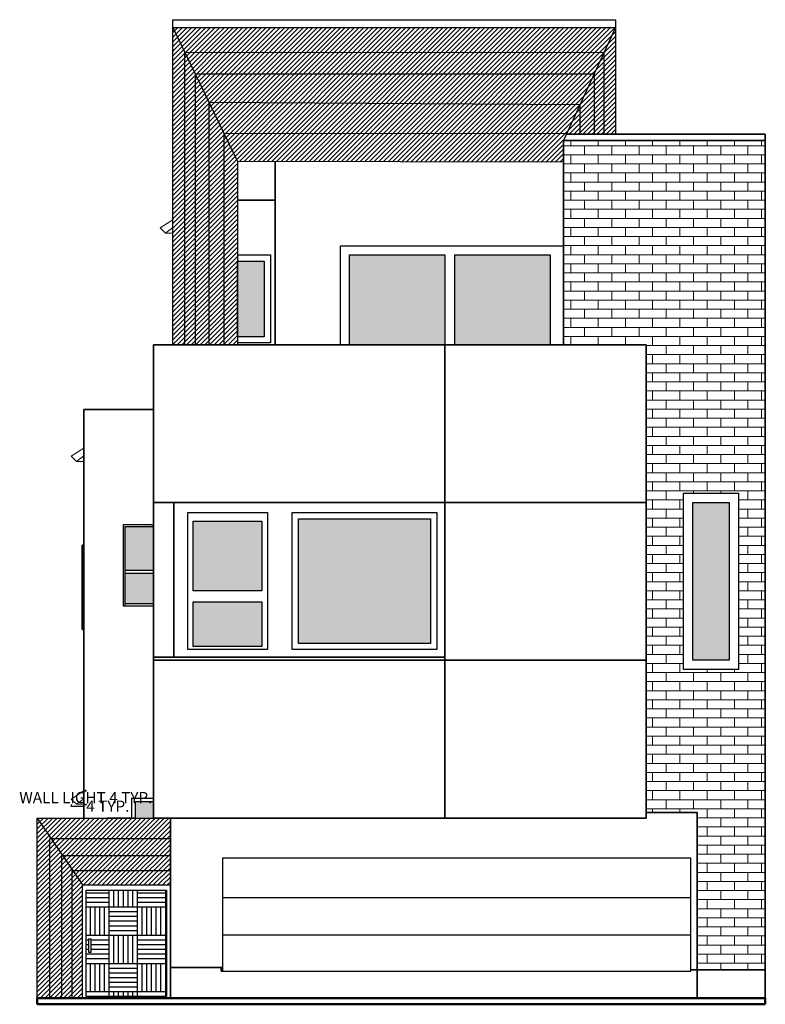
# Model space of a CAD drawing. Units: inches. Extents: x 236 to 476, y 69 to 387.
import ezdxf

# ---------------------------------------------------------------- set-up
doc = ezdxf.new("R2010")
doc.units = ezdxf.units.IN
doc.header["$MEASUREMENT"] = 0
for name, color, linetype, lineweight in [('A-ANNO-DIMS', 2, 'Continuous', 18), ('A-DOOR', 3, 'Continuous', 25), ('A-ELEV', 7, 'Continuous', 35), ('A-ELEV-FIXT', 9, 'Continuous', 18), ('A-ELEV-GRND', 7, 'Continuous', 50), ('A-GLAZ', 4, 'Continuous', 25), ('A-GLAZ-PATT', 251, 'Continuous', 13), ('A-ROOF', 1, 'Continuous', 25), ('A-ROOF-PATT', 8, 'Continuous', 13), ('A-WALL-PATT', 8, 'Continuous', 13)]:
    doc.layers.add(name, color=color, linetype=linetype, lineweight=lineweight)
doc.styles.get("Standard").update_dxf_attribs({"font": 'arial.ttf'})
doc.dimstyles.get("Standard").update_dxf_attribs({"dimtxt": 3.625, "dimasz": 0.18, "dimexe": 0.18, "dimexo": 0.0625, "dimgap": 0.09, "dimtad": 0, "dimtih": 1, "dimtoh": 1, "dimdec": 4, "dimzin": 0, "dimdsep": 46, "dimlunit": 4, "dimtxsty": 'Standard', "dimcen": 0.09, "dimadec": 0, "dimazin": 0, "dimtfac": 1, "dimtdec": 4, "dimtofl": 0, "dimtmove": 0, "dimatfit": 3, "dimfxl": 1, "dimtolj": 1, "dimtzin": 0, "dimarcsym": 0})

# ---------------------------------------------------------------- blocks, each defined once
blk = doc.blocks.new('WALL-LIGHT')
for p, q in [((0, 1.66), (4.13, 4.28)), ((1.8, 0), (0, 1.66)), ((4.13, 1.79), (1.8, 0)), ((1.8, 0), (4.13, 0))]:
    blk.add_line(p, q)
blk = doc.blocks.new('*D2')
at = {"layer": 'A-ANNO-DIMS', "color": 0, "lineweight": -2, "transparency": 16777216}
for p, q in [((256.36, 137.76), (257.12, 137.76)), ((256.94, 137.94), (256.94, 138.12)), ((256.36, 133.48), (257.12, 133.48)), ((256.94, 133.3), (256.94, 133.12))]:
    blk.add_line(p, q, dxfattribs=at)
at = {"layer": 'A-ANNO-DIMS', "color": 0, "transparency": 16777216}
for points in [[(256.91, 137.94), (256.97, 137.94), (256.94, 137.76)], [(256.91, 133.3), (256.97, 133.3), (256.94, 133.48)]]:
    blk.add_solid(points, dxfattribs=at)
at = {"layer": 'Defpoints', "color": 0, "transparency": 16777216}
for p in [(256.29, 137.76), (256.94, 137.76), (256.29, 133.48)]:
    blk.add_point(p, dxfattribs=at)
at = {"layer": 'A-ANNO-DIMS', "color": 0, "transparency": 16777216, "insert": (256.94, 135.62), "char_height": 3.625, "attachment_point": 5}
blk.add_mtext('\\A1;WALL LIGHT 4 TYP.', dxfattribs=at)
blk = doc.blocks.new('*D3')
at = {"layer": 'A-ANNO-DIMS', "color": 0, "lineweight": -2, "transparency": 16777216}
for p, q in [((252.16, 133.42), (252.16, 132.66)), ((252.34, 132.84), (256.11, 132.84)), ((256.29, 133.42), (256.29, 132.66)), ((256.29, 132.84), (256.47, 132.84))]:
    blk.add_line(p, q, dxfattribs=at)
at = {"layer": 'A-ANNO-DIMS', "color": 0, "transparency": 16777216}
for points in [[(252.34, 132.87), (252.34, 132.81), (252.16, 132.84)], [(256.11, 132.87), (256.11, 132.81), (256.29, 132.84)]]:
    blk.add_solid(points, dxfattribs=at)
at = {"layer": 'Defpoints', "color": 0, "transparency": 16777216}
for p in [(252.16, 133.48), (256.29, 133.48), (256.29, 132.84)]:
    blk.add_point(p, dxfattribs=at)
at = {"layer": 'A-ANNO-DIMS', "color": 0, "transparency": 16777216, "insert": (264.05, 132.84), "char_height": 3.625, "attachment_point": 5}
blk.add_mtext('\\A1;4 TYP.', dxfattribs=at)

msp = doc.modelspace()

# ---------------------------------------------------------------- hatches: boundary and pattern name
at = {"layer": 'A-DOOR'}
h = msp.add_hatch(dxfattribs=at)
h.set_pattern_fill('AR-PARQ1', color=256, scale=0.76)
h.paths.add_polyline_path([(283.03, 105.74), (257.04, 105.74), (257.04, 71.42), (283.03, 71.42)])
h.paths.add_polyline_path([(258.54, 89.96), (258.54, 85.61), (257.9, 85.61), (257.9, 89.96)], flags=16)
at = {"layer": 'A-GLAZ-PATT'}
h = msp.add_hatch(color=256, dxfattribs=at)
h.dxf.hatch_style = 1
h.paths.add_polyline_path([(372.93, 310.89), (342.13, 310.89), (342.13, 281.89), (372.93, 281.89)])
h.paths.add_polyline_path([(406.95, 310.89), (376.14, 310.89), (376.14, 281.89), (406.95, 281.89)])
h.paths.add_polyline_path([(368.29, 225.67), (325.59, 225.67), (325.59, 185.43), (368.29, 185.43)])
h.paths.add_polyline_path([(464.7, 230.94), (452.98, 230.94), (452.98, 179.98), (464.7, 179.98)])
h.paths.add_polyline_path([(314.54, 308.89), (305.89, 308.89), (305.89, 284.48), (314.54, 284.48)])
h.paths.add_polyline_path([(313.79, 224.94), (291.63, 224.94), (291.63, 202.39), (313.79, 202.39)])
h.paths.add_polyline_path([(313.79, 198.83), (291.63, 198.83), (291.63, 184.47), (313.79, 184.47)])
h.paths.add_polyline_path([(278.79, 223.2), (269.55, 223.2), (269.55, 209.06), (278.79, 209.06)])
h.paths.add_polyline_path([(278.79, 208.06), (269.55, 208.06), (269.55, 198.34), (278.79, 198.34)])
h.paths.add_polyline_path([(278.79, 134.31), (272.98, 134.31), (272.98, 129.02), (278.79, 129.02)])
at = {"layer": 'A-ROOF-PATT'}
h = msp.add_hatch(dxfattribs=at)
h.set_pattern_fill('ANSI31', color=256, scale=8.5)
h.paths.add_polyline_path([(245.32, 122.42), (245.67, 122.42), (241.2, 129.02), (241.2, 70.86), (245.32, 70.86)])
h.paths.add_polyline_path([(284.25, 129.02), (241.2, 129.02), (245.67, 122.42), (284.25, 122.42)])
h.paths.add_polyline_path([(284.25, 122.42), (245.67, 122.42), (249.39, 116.94), (284.25, 116.94)])
h.paths.add_polyline_path([(249.2, 116.94), (249.39, 116.94), (245.67, 122.42), (245.32, 122.42), (245.32, 70.86), (249.2, 70.86)])
h.paths.add_polyline_path([(252.56, 112.06), (252.71, 112.06), (249.39, 116.94), (249.2, 116.94), (249.2, 70.86), (252.56, 70.86)])
h.paths.add_polyline_path([(284.25, 116.94), (249.39, 116.94), (252.71, 112.06), (284.25, 112.06)])
h.paths.add_polyline_path([(284.25, 112.06), (252.71, 112.06), (255.87, 107.4), (284.25, 107.4)])
h.paths.add_polyline_path([(255.87, 107.4), (252.71, 112.06), (252.56, 112.06), (252.56, 70.86), (255.87, 70.86)])
h.paths.add_polyline_path([(411.16, 347.89), (412.27, 350.27), (301.56, 350.08), (305.89, 341.12), (411.16, 340.89)])
h.paths.add_polyline_path([(416.5, 359.44), (296.66, 360.24), (301.56, 350.08), (412.27, 350.27)])
h.paths.add_polyline_path([(421.09, 369.37), (292.24, 369.37), (296.66, 360.24), (416.5, 359.44)])
h.paths.add_polyline_path([(296.66, 360.24), (292.24, 369.37), (292.24, 281.89), (296.66, 281.89)])
h.paths.add_polyline_path([(292.24, 369.37), (288.84, 376.4), (288.84, 281.89), (292.24, 281.89)])
h.paths.add_polyline_path([(288.84, 376.4), (285.02, 384.32), (285.02, 281.89), (288.84, 281.89)])
h.paths.add_polyline_path([(301.56, 350.08), (296.66, 360.24), (296.66, 281.89), (301.56, 281.89)])
h.paths.add_polyline_path([(305.89, 341.12), (301.56, 350.08), (301.56, 281.89), (305.89, 281.89)])
h.paths.add_polyline_path([(424.28, 376.28), (288.84, 376.4), (292.24, 369.37), (421.09, 369.37)])
h.paths.add_polyline_path([(427.99, 384.32), (285.02, 384.32), (288.84, 376.4), (424.28, 376.28)])
h.paths.add_polyline_path([(421.09, 369.37), (416.5, 359.44), (416.5, 349.89), (421.09, 349.89)])
h.paths.add_polyline_path([(416.5, 359.44), (412.27, 350.27), (412.09, 349.89), (416.5, 349.89)])
h.paths.add_polyline_path([(424.28, 376.28), (421.09, 369.37), (421.09, 349.89), (424.28, 349.89)])
h.paths.add_polyline_path([(427.99, 384.32), (424.28, 376.28), (424.28, 349.89), (427.99, 349.89)])
at = {"layer": 'A-WALL-PATT'}
h = msp.add_hatch(dxfattribs=at)
h.set_pattern_fill('AR-BRSTD', color=256, scale=1.1)
h.paths.add_polyline_path([(476.39, 347.89), (411.16, 347.89), (411.16, 281.89), (437.86, 281.89), (437.86, 230.94), (437.86, 179.98), (437.86, 130.86), (454.36, 130.86), (454.36, 79.99), (460.17, 79.99), (476.39, 79.99), (476.39, 214.86)])
h.paths.add_polyline_path([(449.98, 233.94), (467.7, 233.94), (467.7, 176.98), (449.98, 176.98)], flags=16)
h.paths.add_polyline_path([(452.98, 230.94), (464.7, 230.94), (464.7, 179.98), (452.98, 179.98)], flags=0)

# ---------------------------------------------------------------- linework, layer by layer
at = {"layer": 'A-DOOR'}
for p, q in [((348.17, 116.03), (301.04, 116.03)), ((301.04, 116.03), (301.04, 79.53)), ((452.36, 116.03), (348.17, 116.03)), ((452.36, 79.53), (452.36, 116.03)), ((301.04, 103.41), (452.36, 103.41)), ((301.04, 91.29), (452.36, 91.29)), ((301.04, 79.53), (452.36, 79.53))]:
    msp.add_line(p, q, dxfattribs=at)
for points in [[(257.04, 105.74), (283.03, 105.74), (283.03, 71.42), (257.04, 71.42)], [(257.9, 89.96), (258.54, 89.96), (258.54, 85.61), (257.9, 85.61)]]:
    msp.add_lwpolyline(points, close=True, dxfattribs=at)
at = {"layer": 'A-ELEV'}
for p, q in [((412.09, 349.89), (476.39, 349.89)), ((476.39, 214.86), (476.39, 349.89)), ((411.16, 347.89), (476.39, 347.89)), ((411.16, 347.89), (411.16, 281.89)), ((318.09, 328.57), (318.12, 341.1)), ((305.89, 328.57), (318.09, 328.57)), ((318.09, 328.57), (318.09, 281.89)), ((372.93, 281.89), (372.93, 129.03)), ((278.79, 260.96), (256.29, 260.96)), ((256.29, 260.96), (256.29, 129.02)), ((285.36, 230.94), (285.36, 180.93)), ((256.29, 217.15), (255.79, 217.15)), ((255.79, 217.15), (255.79, 189.88)), ((256.29, 217.15), (256.29, 217.15)), ((476.39, 70.86), (476.39, 214.86)), ((255.79, 189.88), (255.79, 189.88)), ((255.79, 189.88), (256.29, 189.88)), ((278.79, 180.93), (372.93, 180.93)), ((454.36, 130.86), (437.86, 130.86)), ((454.36, 70.86), (454.36, 130.86)), ((272.98, 129.02), (263.76, 129.02)), ((284.25, 129.03), (284.25, 70.86)), ((301.04, 80.73), (284.25, 80.73)), ((300.62, 80.73), (300.62, 79.53)), ((300.62, 79.53), (301.04, 79.53)), ((460.17, 79.99), (452.36, 79.99)), ((460.17, 79.99), (476.39, 79.99))]:
    msp.add_line(p, q, dxfattribs=at)
for points in [[(278.79, 281.89), (437.86, 281.89), (437.86, 230.94), (278.79, 230.94)], [(278.79, 230.94), (437.86, 230.94), (437.86, 179.98), (278.79, 179.98)], [(278.79, 179.98), (437.86, 179.98), (437.86, 129.03), (278.79, 129.03)]]:
    msp.add_lwpolyline(points, close=True, dxfattribs=at)
at = {"layer": 'A-ELEV-GRND'}
for p, q in [((241.2, 70.86), (460.17, 70.86)), ((241.2, 70.86), (241.2, 68.86)), ((460.17, 70.86), (476.39, 70.86)), ((476.39, 68.86), (476.39, 70.86)), ((241.2, 68.86), (460.17, 68.86)), ((460.17, 68.86), (476.39, 68.86))]:
    msp.add_line(p, q, dxfattribs=at)
at = {"layer": 'A-GLAZ'}
for p, q in [((278.2, 223.68), (268.98, 223.68)), ((268.98, 223.68), (268.98, 197.52)), ((269.55, 223.2), (278.79, 223.2)), ((269.55, 223.2), (269.55, 197.52)), ((278.2, 223.68), (278.79, 223.68)), ((269.55, 209.06), (278.79, 209.06)), ((269.55, 208.06), (278.79, 208.06)), ((268.98, 197.52), (278.79, 197.52)), ((269.55, 198.34), (278.79, 198.34)), ((278.79, 135.35), (271.64, 135.35)), ((271.64, 135.35), (271.64, 129.02)), ((272.98, 129.02), (272.98, 134.31)), ((272.98, 134.31), (278.79, 134.31))]:
    msp.add_line(p, q, dxfattribs=at)
for points in [[(339.15, 313.81), (411.16, 313.81), (411.16, 281.89), (339.15, 281.89)], [(305.89, 308.89), (314.54, 308.89), (314.54, 284.48), (305.89, 284.48)], [(342.13, 310.89), (372.93, 310.89), (372.93, 281.89), (342.13, 281.89)], [(376.14, 310.89), (406.95, 310.89), (406.95, 281.89), (376.14, 281.89)], [(449.98, 233.94), (467.7, 233.94), (467.7, 176.98), (449.98, 176.98)], [(452.98, 230.94), (464.7, 230.94), (464.7, 179.98), (452.98, 179.98)], [(289.86, 227.67), (315.64, 227.67), (315.64, 183.43), (289.86, 183.43)], [(323.59, 227.67), (370.29, 227.67), (370.29, 183.43), (323.59, 183.43)], [(291.63, 224.94), (313.79, 224.94), (313.79, 202.39), (291.63, 202.39)], [(325.59, 225.67), (368.29, 225.67), (368.29, 185.43), (325.59, 185.43)], [(291.63, 198.83), (313.79, 198.83), (313.79, 184.47), (291.63, 184.47)]]:
    msp.add_lwpolyline(points, close=True, dxfattribs=at)
msp.add_lwpolyline([(305.89, 310.89), (316.54, 310.89), (316.54, 282.48), (305.89, 282.48)], dxfattribs=at)
at = {"layer": 'A-ROOF'}
for p, q in [((285.02, 384.32), (285.02, 386.87)), ((285.02, 386.87), (427.99, 386.87)), ((427.99, 386.87), (427.99, 384.32)), ((285.02, 281.89), (285.02, 384.32)), ((285.02, 384.32), (427.99, 384.32)), ((285.02, 384.32), (305.89, 341.12)), ((427.99, 384.32), (411.16, 347.89)), ((427.99, 384.32), (427.99, 349.89)), ((288.84, 376.4), (424.28, 376.28)), ((288.84, 376.4), (288.84, 281.89)), ((424.28, 376.28), (424.28, 349.89)), ((292.24, 369.37), (292.24, 281.89)), ((292.24, 369.37), (421.09, 369.37)), ((421.09, 369.37), (421.09, 349.89)), ((296.66, 360.24), (296.66, 281.89)), ((296.66, 360.24), (416.5, 359.44)), ((416.5, 359.44), (416.5, 349.89)), ((301.56, 350.08), (412.27, 350.27)), ((301.56, 350.08), (301.56, 281.89)), ((411.16, 340.89), (305.89, 341.12)), ((305.89, 341.12), (305.89, 281.89)), ((241.2, 129.02), (255.87, 107.4))]:
    msp.add_line(p, q, dxfattribs=at)
for points in [[(284.25, 70.86), (241.2, 70.86), (241.2, 129.02), (284.25, 129.02)], [(245.32, 122.42), (284.25, 122.42), (284.25, 70.86), (245.32, 70.86)], [(249.2, 116.94), (284.25, 116.94), (284.25, 70.86), (249.2, 70.86)], [(252.56, 112.06), (284.25, 112.06), (284.25, 70.86), (252.56, 70.86)], [(255.87, 107.4), (284.25, 107.4), (284.25, 70.86), (255.87, 70.86)]]:
    msp.add_lwpolyline(points, close=True, dxfattribs=at)

# ---------------------------------------------------------------- block references
at = {"layer": 'A-ELEV-FIXT'}
for p in [(280.89, 317.94), (252.16, 244.22), (252.16, 133.48)]:
    msp.add_blockref('WALL-LIGHT', p, dxfattribs=at)

# ---------------------------------------------------------------- dimensions: what is measured, and where the dimension line sits
at = {"layer": 'A-ANNO-DIMS'}
dim = msp.add_linear_dim(base=(256.94, 137.76), p1=(256.29, 133.48), p2=(256.29, 137.76), angle=90, text='WALL LIGHT <> TYP.', dimstyle='Standard', override={"dimdec": 0, "dimlfac": 1, "dimrnd": 0, "dimzin": 0, "dimdsep": 46, "dimlunit": 2}, dxfattribs=at)
dim.commit()
dim.dimension.update_dxf_attribs({"geometry": '*D2', "text_midpoint": (256.94, 135.62)})
dim = msp.add_linear_dim(base=(256.29, 132.84), p1=(252.16, 133.48), p2=(256.29, 133.48), text='<> TYP.', dimstyle='Standard', override={"dimdec": 0, "dimlfac": 1, "dimrnd": 0, "dimzin": 0, "dimdsep": 46, "dimlunit": 2}, dxfattribs=at)
dim.commit()
dim.dimension.update_dxf_attribs({"geometry": '*D3', "text_midpoint": (264.05, 132.84)})

doc.saveas('drawing.dxf')
